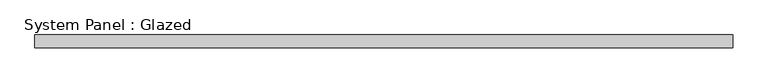
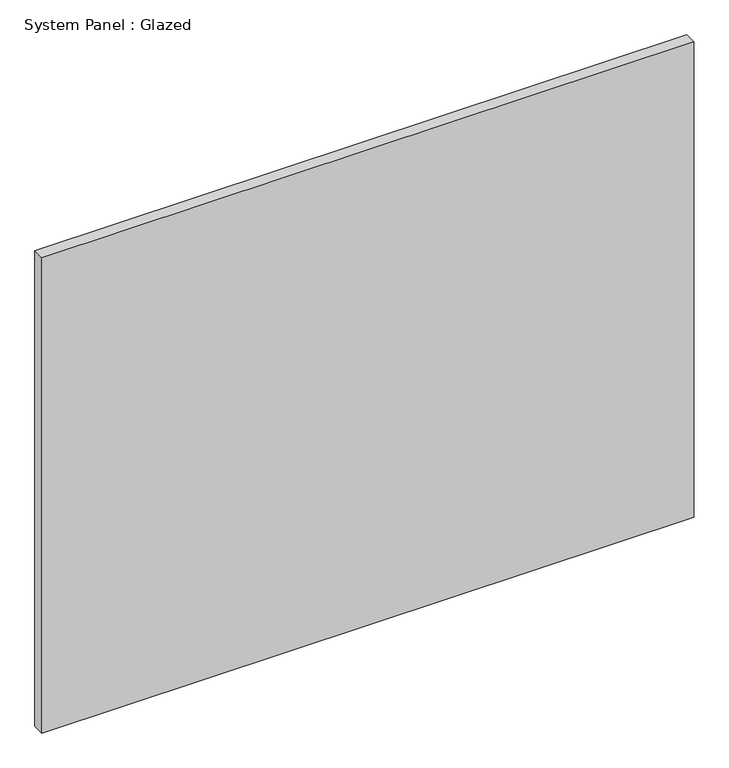
"""IFC4 building model written with IfcOpenShell, lengths in millimetres: plate geometry, System Panel : Glazed."""

from ifc_helpers import new_model, si_unit, origin, origin_with_axes, place, context, project, spatial, polyline, outline, extrude, source, transform, mapped, element, save


def system_panel_glazed_e2854511(model_context):
    return source(origin(), model_context, "Body", "SweptSolid", [
        extrude(outline(polyline([(685.8, 24.5), (-685.8, 24.5), (-685.8, 49.5), (685.8, 49.5), (685.8, 24.5)])), origin_with_axes(), (0.0, 0.0, 1.0), 1057.5402127),
    ])


if __name__ == "__main__":
    model = new_model("IFC4")
    model_context = context("Model", 3, world=origin())
    ifc_project = project(units=[si_unit("LENGTHUNIT", "METRE", prefix="MILLI")], contexts=[model_context])
    site = spatial("IfcSite", under=ifc_project)
    building = spatial("IfcBuilding", under=site)
    placement = place(None, origin())
    system_panel_glazed_shape = system_panel_glazed_e2854511(model_context)
    element("IfcPlate", 1, ObjectType="System Panel : Glazed", at=placement, inside=building, context=model_context, shape_type="MappedRepresentation", body=[
        mapped(system_panel_glazed_shape, transform((0.0, 0.0, 0.0), x_axis=(1.0, 0.0, 0.0), y_axis=(0.0, 1.0, 0.0), z_axis=(0.0, 0.0, 1.0))),
    ])
    save(model, "model.ifc")

# Revit data of these elements
# Type "System Panel : Glazed"
#   Keynote = "H11"
#   Construction Type Id = "GSP4R"
#   Analytic Construction = "1/8 in Pilkington single glazing"
#   Visual Light Transmittance = 0.9
#   Solar Heat Gain Coefficient = 0.86
#   Heat Transfer Coefficient (U) = 6.7069 W/(m²·K)
#   Define Thermal Properties by = 1
# Element 1 (IfcPlate, "System Panel : Glazed")
#   Materials on its faces: "Glass"
# Materials
#   "Glass": class "Glass", colour RGB 0 128 192, transparency 0.9, Description = "Soda Lime Glass", Cost = 0
